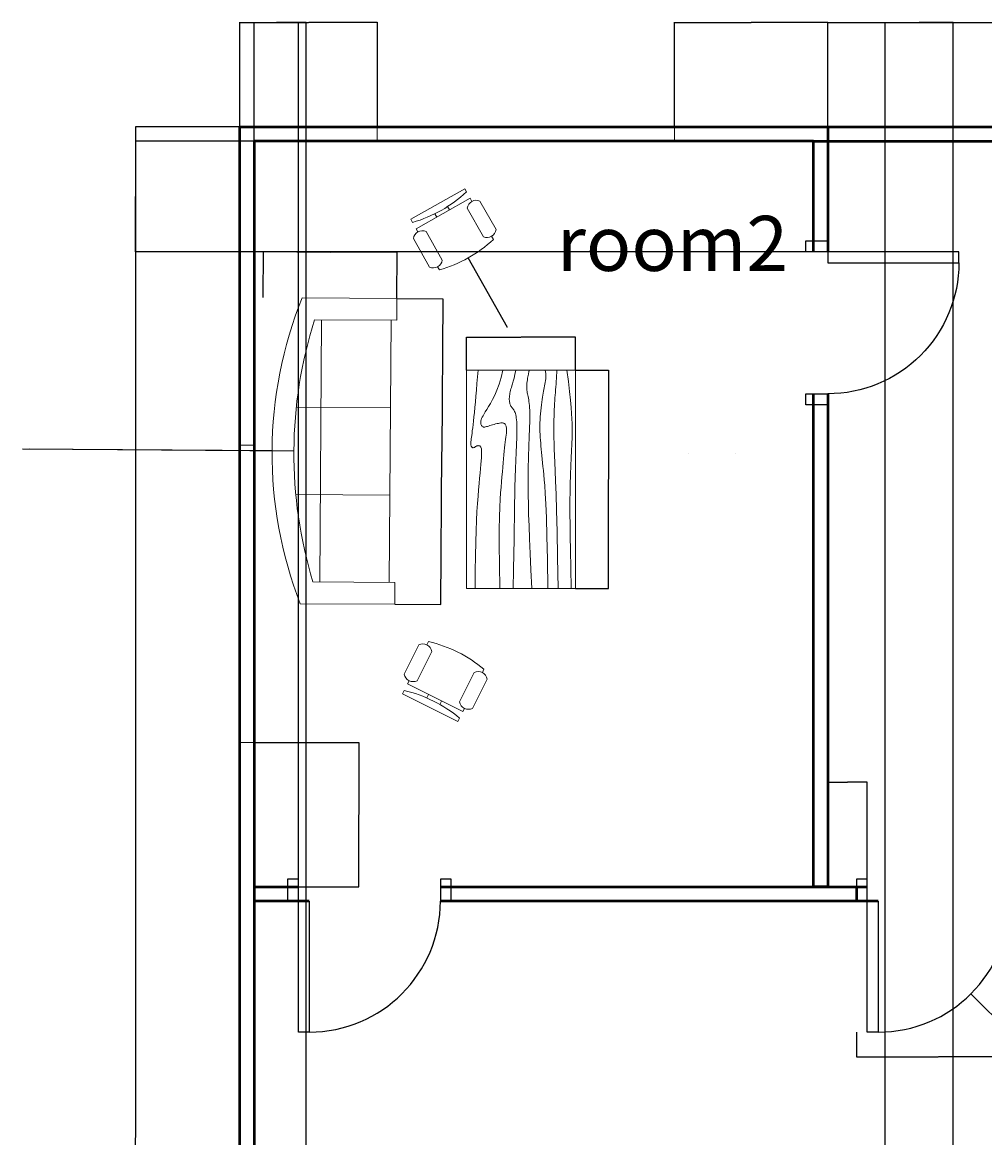
# Model space of a CAD drawing. Units: millimetres. Extents: x 756 to 17937, y 31 to 15590.
# Tile 2 of 6: x 756 to 7469, y 7810 to 15590. Entities that reach past the tile are written whole.
import ezdxf

# ---------------------------------------------------------------- set-up
doc = ezdxf.new("R2010")
doc.units = ezdxf.units.MM
for name, color, linetype, lineweight in [('A-ANNO-DIMS', 2, 'Continuous', 18), ('A-AREA-IDEN', 7, 'Continuous', 25), ('A-DOOR', 3, 'Continuous', 25), ('A-FURN', 8, 'Continuous', 18), ('A-GLAZ', 4, 'Continuous', 18), ('A-WALL', 7, 'Continuous', 50)]:
    doc.layers.add(name, color=color, linetype=linetype, lineweight=lineweight)
doc.styles.get("Standard").update_dxf_attribs({"font": 'arial.ttf'})
doc.dimstyles.get("Standard").update_dxf_attribs({"dimtxt": 0.18, "dimasz": 0.18, "dimexe": 0.18, "dimexo": 0.0625, "dimgap": 0.09, "dimtad": 0, "dimtih": 1, "dimtoh": 1, "dimdec": 4, "dimzin": 0, "dimdsep": 46, "dimtxsty": 'Standard', "dimcen": 0.09, "dimadec": 0, "dimazin": 0, "dimtfac": 1, "dimtdec": 4, "dimtofl": 0, "dimtmove": 0, "dimatfit": 3, "dimfxl": 1, "dimtolj": 1, "dimtzin": 0, "dimarcsym": 0})

# ---------------------------------------------------------------- blocks, each defined once
blk = doc.blocks.new('Sofa - Roundback 7 ft.')
for p, q in [((-12.00002, -32.4421), (-12.00003, -6.5971)), ((11.99997, -32.4421), (11.99998, -6.5971)), ((-36.000027, -34), (-36.000027, -11.4696)), ((35.99998, -34), (35.99998, -11.4696)), ((-35.999844, -13.3819), (35.9998, -13.3819)), ((-36.000027, -32.4421), (35.99998, -32.4421))]:
    blk.add_line(p, q)
for points in [[(-36.000027, -34), (-42.000027, -34), (-42.000027, -8)], [(41.99998, -8), (41.99998, -34), (35.99998, -34)]]:
    blk.add_lwpolyline(points)
for centre, radius, start, end in [((0, -114.25), 114.25, 68.43141, 111.5686), ((-0.00001, -127.1968), 121.1968, 72.72033, 107.2797)]:
    blk.add_arc(centre, radius, start, end)
blk = doc.blocks.new('Table - Rectangular Woodgrain 60 x 30 in.')
for p, q in [((0, 0), (0, -30)), ((60, 0), (0, 0)), ((60, -30), (60, 0)), ((0, -30), (60, -30))]:
    blk.add_line(p, q)
for points in [[(0, -2.4), (4.8155, -2.418), (9.0302, -2.4688), (12.709, -2.5477), (15.9167, -2.65), (18.7181, -2.7711), (21.1781, -2.9063), (23.3616, -3.0508), (25.3333, -3.2), (27.1477, -3.3495), (28.8172, -3.4958), (30.3437, -3.636), (31.7291, -3.7667), (32.9756, -3.8849), (34.0849, -3.9875), (35.059, -4.0714), (35.9, -4.1334), (36.6114, -4.1711), (37.2041, -4.1854), (37.6906, -4.1779), (38.0833, -4.15), (38.3948, -4.1034), (38.6375, -4.0396), (38.8239, -3.9602), (38.9666, -3.8667), (39.0764, -3.7608), (39.1573, -3.6448), (39.2116, -3.521), (39.2416, -3.3917), (39.2498, -3.2593), (39.2385, -3.1261), (39.21, -2.9944), (39.1666, -2.8667), (39.111, -2.7447), (39.0468, -2.6281), (38.978, -2.5163), (38.9083, -2.4083), (38.8418, -2.3035), (38.7823, -2.201), (38.7337, -2.1001), (38.7, -2), (38.6844, -1.9003), (38.6875, -1.8021), (38.7094, -1.707), (38.75, -1.6167), (38.8094, -1.5326), (38.8875, -1.4563), (38.9844, -1.3893), (39.1, -1.3333), (39.2351, -1.2896), (39.3937, -1.2583), (39.5804, -1.2396), (39.8, -1.2333), (40.057, -1.2396), (40.3562, -1.2583), (40.7023, -1.2896), (41.1, -1.3333), (41.5547, -1.3895), (42.0755, -1.4573), (42.6721, -1.5361), (43.3542, -1.625), (44.1316, -1.7233), (45.014, -1.8302), (46.0114, -1.9449), (47.1333, -2.0667), (48.3862, -2.1947), (49.7625, -2.3281), (51.2513, -2.4663), (52.8416, -2.6083), (54.5226, -2.7535), (56.2833, -2.9011), (58.1127, -3.0501), (60, -3.2)], [(0, -9.2), (6.5759, -9.0858), (11.9385, -9.0365), (16.2527, -9.0418), (19.6833, -9.0917), (22.3952, -9.1759), (24.5531, -9.2844), (26.322, -9.4069), (27.8666, -9.5333), (29.3241, -9.6553), (30.7203, -9.7719), (32.0532, -9.8837), (33.3208, -9.9917), (34.5213, -10.0965), (35.6526, -10.199), (36.7128, -10.2999), (37.7, -10.4), (38.6129, -10.4996), (39.4531, -10.5969), (40.223, -10.6895), (40.925, -10.775), (41.5613, -10.8512), (42.1344, -10.9156), (42.6465, -10.966), (43.1, -11), (43.4976, -11.0158), (43.8437, -11.0136), (44.143, -10.9942), (44.4, -10.9583), (44.6195, -10.9069), (44.8062, -10.8406), (44.9648, -10.7603), (45.1, -10.6667), (45.2155, -10.5598), (45.3114, -10.4365), (45.3871, -10.2929), (45.4416, -10.125), (45.4743, -9.929), (45.4844, -9.7011), (45.4709, -9.4371), (45.4333, -9.1333), (45.3716, -8.7883), (45.2896, -8.4104), (45.1919, -8.0107), (45.0833, -7.6), (44.9685, -7.1893), (44.8521, -6.7896), (44.7388, -6.4117), (44.6333, -6.0667), (44.54, -5.7628), (44.4614, -5.4979), (44.4001, -5.2675), (44.3583, -5.0667), (44.3384, -4.8909), (44.3427, -4.7354), (44.3736, -4.5956), (44.4333, -4.4667), (44.5236, -4.3453), (44.6427, -4.2333), (44.7884, -4.1339), (44.9583, -4.05), (45.1501, -3.9849), (45.3614, -3.9417), (45.59, -3.9234), (45.8333, -3.9333), (46.0915, -3.9749), (46.3734, -4.0531), (46.6906, -4.1736), (47.0542, -4.3417), (47.4756, -4.5629), (47.9661, -4.8427), (48.5372, -5.1866), (49.2, -5.6), (49.9676, -6.0844), (50.8594, -6.625), (51.8965, -7.2031), (53.1, -7.8), (54.491, -8.3969), (56.0906, -8.975), (57.9199, -9.5156), (60, -10)], [(0, -12.8), (5.1847, -12.9322), (9.6213, -13.0323), (13.3963, -13.1059), (16.5958, -13.1583), (19.3063, -13.1952), (21.614, -13.2219), (23.6054, -13.2439), (25.3666, -13.2667), (26.9728, -13.2947), (28.4531, -13.3281), (29.8256, -13.3663), (31.1083, -13.4083), (32.3191, -13.4535), (33.476, -13.501), (34.597, -13.5501), (35.7, -13.6), (36.7984, -13.6497), (37.8875, -13.6979), (38.9578, -13.743), (40, -13.7833), (41.0047, -13.8174), (41.9625, -13.8438), (42.864, -13.8607), (43.7, -13.8667), (44.4631, -13.8604), (45.1552, -13.8417), (45.7801, -13.8104), (46.3416, -13.7667), (46.8439, -13.7104), (47.2906, -13.6417), (47.6858, -13.5604), (48.0333, -13.4667), (48.3375, -13.3608), (48.6042, -13.2448), (48.8396, -13.121), (49.05, -12.9917), (49.2417, -12.8593), (49.4208, -12.7261), (49.5937, -12.5944), (49.7667, -12.4667), (49.9452, -12.3451), (50.1323, -12.2313), (50.3303, -12.1268), (50.5416, -12.0333), (50.7686, -11.9524), (51.0135, -11.8854), (51.2788, -11.8341), (51.5666, -11.8), (51.8785, -11.7843), (52.2116, -11.7865), (52.562, -11.8059), (52.926, -11.8417), (53.2998, -11.8931), (53.6795, -11.9594), (54.0614, -12.0397), (54.4416, -12.1333), (54.8223, -12.2401), (55.2293, -12.3625), (55.6942, -12.5037), (56.2489, -12.6667), (56.9251, -12.8547), (57.7545, -13.0708), (58.7689, -13.3182), (60, -13.6)], [(0, -18), (5.124, -17.7273), (9.6609, -17.5057), (13.6705, -17.3303), (17.2125, -17.1958), (20.3467, -17.0973), (23.1328, -17.0297), (25.6307, -16.9878), (27.9, -16.9667), (29.9928, -16.9617), (31.9302, -16.9703), (33.7254, -16.9907), (35.3917, -17.0208), (36.9423, -17.0588), (38.3906, -17.1026), (39.7499, -17.1503), (41.0333, -17.2), (42.2519, -17.2496), (43.4073, -17.2969), (44.4986, -17.3395), (45.525, -17.375), (46.4858, -17.4012), (47.3802, -17.4156), (48.2074, -17.416), (48.9667, -17.4), (49.6583, -17.3662), (50.2872, -17.3167), (50.8595, -17.2547), (51.3812, -17.1833), (51.8584, -17.1057), (52.2971, -17.025), (52.7034, -16.9443), (53.0833, -16.8667), (53.443, -16.7951), (53.789, -16.7313), (54.128, -16.6768), (54.4666, -16.6334), (54.8115, -16.6024), (55.1693, -16.5854), (55.5465, -16.5841), (55.95, -16.6), (56.3828, -16.6337), (56.8346, -16.6823), (57.2915, -16.7418), (57.7396, -16.8084), (58.165, -16.878), (58.5539, -16.9469), (58.8924, -17.0111), (59.1666, -17.0667), (59.3679, -17.1107), (59.5078, -17.1438), (59.6032, -17.1675), (59.6708, -17.1833), (59.7275, -17.193), (59.7901, -17.1979), (59.8753, -17.1998), (60, -17.2)], [(0, -22.4), (8.0098, -22.2501), (14.4094, -22.1011), (19.4168, -21.9535), (23.25, -21.8083), (26.1269, -21.6663), (28.2656, -21.5281), (29.884, -21.3947), (31.2, -21.2667), (32.3967, -21.1448), (33.5172, -21.0292), (34.5697, -20.9198), (35.5625, -20.8167), (36.5037, -20.7198), (37.4015, -20.6292), (38.2642, -20.5448), (39.1, -20.4667), (39.9164, -20.3951), (40.7187, -20.3313), (41.5117, -20.2768), (42.3, -20.2333), (43.0883, -20.2024), (43.8812, -20.1854), (44.6836, -20.1841), (45.5, -20.2), (46.3328, -20.234), (47.1747, -20.2844), (48.0163, -20.3488), (48.8479, -20.425), (49.66, -20.5106), (50.4429, -20.6031), (51.1872, -20.7004), (51.8833, -20.8), (52.5246, -20.8999), (53.1166, -20.9995), (53.6681, -21.0983), (54.1875, -21.1958), (54.6834, -21.2919), (55.1646, -21.3859), (55.6394, -21.4777), (56.1167, -21.5667), (56.6028, -21.6515), (57.0961, -21.7266), (57.5929, -21.7852), (58.0896, -21.8208), (58.5823, -21.8268), (59.0674, -21.7964), (59.5412, -21.723), (60, -21.6)], [(0, -25.2), (8.6355, -25.0504), (15.7026, -24.9031), (21.4049, -24.7606), (25.9458, -24.625), (29.529, -24.4988), (32.3578, -24.3844), (34.6359, -24.284), (36.5667, -24.2), (38.3213, -24.1341), (39.9417, -24.0854), (41.437, -24.0523), (42.8167, -24.0333), (44.0901, -24.0268), (45.2667, -24.0313), (46.3557, -24.0451), (47.3667, -24.0667), (48.309, -24.0947), (49.1928, -24.1287), (50.0284, -24.168), (50.826, -24.2125), (51.5959, -24.2617), (52.3483, -24.3151), (53.0935, -24.3725), (53.8417, -24.4334), (54.6009, -24.497), (55.3699, -24.561), (56.1454, -24.6226), (56.9239, -24.6792), (57.7021, -24.7279), (58.4764, -24.7662), (59.2435, -24.7911), (60, -24.8)], [(0, -28.8), (5.6867, -28.6681), (10.45, -28.5698), (14.407, -28.5012), (17.675, -28.4584), (20.3711, -28.4374), (22.6125, -28.4344), (24.5164, -28.4455), (26.2, -28.4667), (27.762, -28.4947), (29.2276, -28.5281), (30.6033, -28.5663), (31.8958, -28.6084), (33.1118, -28.6535), (34.2578, -28.7011), (35.3405, -28.7501), (36.3666, -28.8), (37.3443, -28.8497), (38.288, -28.8974), (39.2137, -28.9412), (40.1375, -28.9792), (41.0753, -29.0093), (42.0432, -29.0297), (43.0572, -29.0384), (44.1333, -29.0333), (45.2936, -29.0114), (46.5843, -28.9641), (48.0579, -28.8816), (49.7666, -28.7542), (51.7629, -28.5721), (54.0989, -28.3255), (56.8272, -28.0048), (60, -27.6)]]:
    blk.add_lwpolyline(points)
blk = doc.blocks.new('Chair - Desk')
for p, q in [((-8.5, 0), (-8.5, -1)), ((-8.5, 0), (8.5, 0)), ((8.5, 0), (8.5, -1)), ((-8.5, -3), (-8.5, -4)), ((-8.5, -3), (8.5, -3)), ((-2, -3), (-2, -1.9355)), ((2, -1.9576), (2, -3)), ((8.5, -3), (8.5, -4)), ((-10.5, -5), (-10.5, -14)), ((-6.5, -14), (-6.5, -5)), ((6.5, -5), (6.5, -14)), ((10.5, -14), (10.5, -5)), ((-8.5, -15), (-8.5, -16)), ((8.5, -15), (8.5, -16))]:
    blk.add_line(p, q)
for centre, radius, start, end in [((0, 34.625), 36.625, 256.5803, 283.4197), ((-8.5, -6.5), 2.5, 36.8699, 143.1301), ((8.5, -6.5), 2.5, 36.8699, 143.1301), ((-8.5, -12.5), 2.5, 216.8699, 323.1301), ((8.5, -12.5), 2.5, 216.8699, 323.1301), ((0, 19.625), 36.625, 256.5803, 283.4197)]:
    blk.add_arc(centre, radius, start, end)
blk = doc.blocks.new('DOOR-SINGLE-914')
for p, q in [((76.2, 1066.8), (0, 1066.8)), ((0, 1066.8), (0, 914.4)), ((76.2, 914.4), (76.2, 1066.8)), ((1143, 1066.8), (1066.8, 1066.8)), ((1066.8, 1066.8), (1066.8, 914.4)), ((1143, 914.4), (1143, 1066.8)), ((0, 914.4), (76.2, 914.4)), ((76.2, 914.4), (152.4, 914.4)), ((76.2, 0), (76.2, 914.4)), ((152.4, 914.4), (152.4, 0)), ((1066.8, 914.4), (1143, 914.4)), ((152.4, 0), (76.2, 0))]:
    blk.add_line(p, q)
blk.add_arc((152.4, 914.4), 914.4, 270, 0)
blk = doc.blocks.new('WIN-2073')
for p, q in [((0, 100), (0, 0)), ((2072.9, 100), (0, 100)), ((2072.9, 0), (2072.9, 100)), ((0, 0), (2072.9, 0))]:
    blk.add_line(p, q)
blk = doc.blocks.new('*D15')
at = {"layer": 'A-ANNO-DIMS', "color": 0, "lineweight": -2, "transparency": 16777216}
for p, q in [((6574.2, 8546.1), (6574.2, 8374.6)), ((7717.2, 8546.1), (7717.2, 8374.6)), ((6574.4, 8374.8), (7144.1, 8374.8)), ((7717, 8374.8), (7147.3, 8374.8))]:
    blk.add_line(p, q, dxfattribs=at)
at = {"layer": 'A-ANNO-DIMS', "color": 0, "transparency": 16777216}
for points in [[(6574.4, 8374.8), (6574.4, 8374.7), (6574.2, 8374.8)], [(7717, 8374.8), (7717, 8374.7), (7717.2, 8374.8)]]:
    blk.add_solid(points, dxfattribs=at)
at = {"layer": 'Defpoints', "color": 0, "transparency": 16777216}
for p in [(6574.2, 8546.2), (7717.2, 8546.2), (7717.2, 8374.8)]:
    blk.add_point(p, dxfattribs=at)
at = {"layer": 'A-ANNO-DIMS', "color": 0, "transparency": 16777216, "insert": (7145.7, 8374.8), "char_height": 0.18, "attachment_point": 5}
blk.add_mtext('\\A1;SINGLE DOOR 1143 TYP.', dxfattribs=at)
blk = doc.blocks.new('*D27')
at = {"layer": 'A-ANNO-DIMS', "color": 0, "lineweight": -2, "transparency": 16777216}
for p, q in [((3368.6, 13664), (3688.7, 13661.9)), ((3688.6, 13661.7), (3681.7, 12595.3)), ((3674.8, 11528.5), (3681.7, 12594.9)), ((3354.8, 11530.4), (3675, 11528.3))]:
    blk.add_line(p, q, dxfattribs=at)
at = {"layer": 'A-ANNO-DIMS', "color": 0, "transparency": 16777216}
for points in [[(3688.5, 13661.7), (3688.6, 13661.7), (3688.6, 13661.9)], [(3674.8, 11528.5), (3674.8, 11528.5), (3674.8, 11528.3)]]:
    blk.add_solid(points, dxfattribs=at)
at = {"layer": 'Defpoints', "color": 0, "transparency": 16777216}
for p in [(3368.5, 13664), (3688.6, 13661.9), (3354.8, 11530.4)]:
    blk.add_point(p, dxfattribs=at)
at = {"layer": 'A-ANNO-DIMS', "color": 0, "transparency": 16777216, "insert": (3681.7, 12595.1), "char_height": 0.18, "attachment_point": 5}
blk.add_mtext('\\A1;SOFA 2134', dxfattribs=at)
blk = doc.blocks.new('*D28')
at = {"layer": 'A-ANNO-DIMS', "color": 0, "lineweight": -2, "transparency": 16777216}
for p, q in [((2437.2, 13670), (2439.3, 13990.2)), ((2439.4, 13990), (2904.7, 13987)), ((3370.4, 13984), (2905.2, 13987)), ((3368.5, 13664), (3370.6, 13984.2))]:
    blk.add_line(p, q, dxfattribs=at)
at = {"layer": 'A-ANNO-DIMS', "color": 0, "transparency": 16777216}
for points in [[(2439.4, 13990), (2439.4, 13990), (2439.3, 13990)], [(3370.4, 13984), (3370.4, 13984), (3370.6, 13984)]]:
    blk.add_solid(points, dxfattribs=at)
at = {"layer": 'Defpoints', "color": 0, "transparency": 16777216}
for p in [(2439.3, 13990), (2437.2, 13670), (3368.5, 13664)]:
    blk.add_point(p, dxfattribs=at)
at = {"layer": 'A-ANNO-DIMS', "color": 0, "transparency": 16777216, "insert": (2904.9, 13987), "char_height": 0.18, "attachment_point": 5}
blk.add_mtext('\\A1;931', dxfattribs=at)
blk = doc.blocks.new('*D29')
at = {"layer": 'A-ANNO-DIMS', "color": 0, "lineweight": -2, "transparency": 16777216}
for p, q in [((4616, 13164.1), (4844.7, 13164.1)), ((4844.5, 13163.9), (4844.5, 12402.3)), ((4844.5, 11640.3), (4844.5, 12401.9)), ((4616, 11640.1), (4844.7, 11640.1))]:
    blk.add_line(p, q, dxfattribs=at)
at = {"layer": 'A-ANNO-DIMS', "color": 0, "transparency": 16777216}
for points in [[(4844.5, 13163.9), (4844.5, 13163.9), (4844.5, 13164.1)], [(4844.5, 11640.3), (4844.5, 11640.3), (4844.5, 11640.1)]]:
    blk.add_solid(points, dxfattribs=at)
at = {"layer": 'Defpoints', "color": 0, "transparency": 16777216}
for p in [(4615.9, 13164.1), (4844.5, 13164.1), (4615.9, 11640.1)]:
    blk.add_point(p, dxfattribs=at)
at = {"layer": 'A-ANNO-DIMS', "color": 0, "transparency": 16777216, "insert": (4844.5, 12402.1), "char_height": 0.18, "attachment_point": 5}
blk.add_mtext('\\A1;LOW TABLE 1524', dxfattribs=at)
blk = doc.blocks.new('*D30')
at = {"layer": 'A-ANNO-DIMS', "color": 0, "lineweight": -2, "transparency": 16777216}
for p, q in [((3853.9, 13164.1), (3853.9, 13392.9)), ((3854.1, 13392.7), (4234.6, 13392.7)), ((4615.7, 13392.7), (4235.2, 13392.7)), ((4615.9, 13164.1), (4615.9, 13392.9))]:
    blk.add_line(p, q, dxfattribs=at)
at = {"layer": 'A-ANNO-DIMS', "color": 0, "transparency": 16777216}
for points in [[(3854.1, 13392.7), (3854.1, 13392.6), (3853.9, 13392.7)], [(4615.7, 13392.7), (4615.7, 13392.6), (4615.9, 13392.7)]]:
    blk.add_solid(points, dxfattribs=at)
at = {"layer": 'Defpoints', "color": 0, "transparency": 16777216}
for p in [(3853.9, 13392.7), (3853.9, 13164.1), (4615.9, 13164.1)]:
    blk.add_point(p, dxfattribs=at)
at = {"layer": 'A-ANNO-DIMS', "color": 0, "transparency": 16777216, "insert": (4234.9, 13392.7), "char_height": 0.18, "attachment_point": 5}
blk.add_mtext('\\A1;762', dxfattribs=at)
blk = doc.blocks.new('*D44')
at = {"layer": 'A-ANNO-DIMS', "color": 0, "lineweight": -2, "transparency": 16777216}
for p, q in [((2274.1, 14860.2), (1544.7, 14860.2)), ((1544.9, 14860), (1544.9, 7810.4)), ((1544.9, 760.4), (1544.9, 7810)), ((2274.1, 760.2), (1544.7, 760.2))]:
    blk.add_line(p, q, dxfattribs=at)
at = {"layer": 'A-ANNO-DIMS', "color": 0, "transparency": 16777216}
for points in [[(1544.8, 14860), (1544.9, 14860), (1544.9, 14860.2)], [(1544.8, 760.4), (1544.9, 760.4), (1544.9, 760.2)]]:
    blk.add_solid(points, dxfattribs=at)
at = {"layer": 'Defpoints', "color": 0, "transparency": 16777216}
for p in [(1544.9, 14860.2), (2274.1, 14860.2), (2274.1, 760.2)]:
    blk.add_point(p, dxfattribs=at)
at = {"layer": 'A-ANNO-DIMS', "color": 0, "transparency": 16777216, "insert": (1544.9, 7810.2), "char_height": 0.18, "attachment_point": 5}
blk.add_mtext('\\A1;14100', dxfattribs=at)
blk = doc.blocks.new('*D53')
at = {"layer": 'A-ANNO-DIMS', "color": 0, "lineweight": -2, "transparency": 16777216}
for p, q in [((2274.1, 14860.2), (2274.1, 15589.6)), ((2274.3, 15589.4), (2753, 15589.4)), ((3232.4, 15589.4), (2753.7, 15589.4)), ((3232.6, 14860.2), (3232.6, 15589.6))]:
    blk.add_line(p, q, dxfattribs=at)
at = {"layer": 'A-ANNO-DIMS', "color": 0, "transparency": 16777216}
for points in [[(2274.3, 15589.5), (2274.3, 15589.4), (2274.1, 15589.4)], [(3232.4, 15589.5), (3232.4, 15589.4), (3232.6, 15589.4)]]:
    blk.add_solid(points, dxfattribs=at)
at = {"layer": 'Defpoints', "color": 0, "transparency": 16777216}
for p in [(3232.6, 15589.4), (2274.1, 14860.2), (3232.6, 14860.2)]:
    blk.add_point(p, dxfattribs=at)
at = {"layer": 'A-ANNO-DIMS', "color": 0, "transparency": 16777216, "insert": (2753.3, 15589.4), "char_height": 0.18, "attachment_point": 5}
blk.add_mtext('\\A1;958.5', dxfattribs=at)
blk = doc.blocks.new('*D54')
at = {"layer": 'A-ANNO-DIMS', "color": 0, "lineweight": -2, "transparency": 16777216}
for p, q in [((5305.5, 14860.2), (5305.5, 15589.6)), ((5305.7, 15589.4), (5839.3, 15589.4)), ((6373.9, 15589.4), (5840.3, 15589.4)), ((6374.1, 14860.2), (6374.1, 15589.6))]:
    blk.add_line(p, q, dxfattribs=at)
at = {"layer": 'A-ANNO-DIMS', "color": 0, "transparency": 16777216}
for points in [[(5305.7, 15589.5), (5305.7, 15589.4), (5305.5, 15589.4)], [(6373.9, 15589.5), (6373.9, 15589.4), (6374.1, 15589.4)]]:
    blk.add_solid(points, dxfattribs=at)
at = {"layer": 'Defpoints', "color": 0, "transparency": 16777216}
for p in [(6374.1, 15589.4), (5305.5, 14860.2), (6374.1, 14860.2)]:
    blk.add_point(p, dxfattribs=at)
at = {"layer": 'A-ANNO-DIMS', "color": 0, "transparency": 16777216, "insert": (5839.8, 15589.4), "char_height": 0.18, "attachment_point": 5}
blk.add_mtext('\\A1;1068.6', dxfattribs=at)
blk = doc.blocks.new('*D55')
at = {"layer": 'A-ANNO-DIMS', "color": 0, "lineweight": -2, "transparency": 16777216}
for p, q in [((6374.1, 14860.2), (6374.1, 15589.6)), ((6374.3, 15589.4), (7637, 15589.4)), ((8900.6, 15589.4), (7637.9, 15589.4)), ((8900.8, 14860.2), (8900.8, 15589.6))]:
    blk.add_line(p, q, dxfattribs=at)
at = {"layer": 'A-ANNO-DIMS', "color": 0, "transparency": 16777216}
for points in [[(6374.3, 15589.5), (6374.3, 15589.4), (6374.1, 15589.4)], [(8900.6, 15589.5), (8900.6, 15589.4), (8900.8, 15589.4)]]:
    blk.add_solid(points, dxfattribs=at)
at = {"layer": 'Defpoints', "color": 0, "transparency": 16777216}
for p in [(8900.8, 15589.4), (6374.1, 14860.2), (8900.8, 14860.2)]:
    blk.add_point(p, dxfattribs=at)
at = {"layer": 'A-ANNO-DIMS', "color": 0, "transparency": 16777216, "insert": (7637.4, 15589.4), "char_height": 0.18, "attachment_point": 5}
blk.add_mtext('\\A1;2526.6', dxfattribs=at)
blk = doc.blocks.new('*D63')
at = {"layer": 'A-ANNO-DIMS', "color": 0, "lineweight": -2, "transparency": 16777216}
for p, q in [((2374.1, 860.2), (2374.1, 15589.6)), ((2374.3, 15589.4), (2554.6, 15589.4)), ((2735.7, 15589.4), (2555.4, 15589.4)), ((2735.9, 760.2), (2735.9, 15589.6))]:
    blk.add_line(p, q, dxfattribs=at)
at = {"layer": 'A-ANNO-DIMS', "color": 0, "transparency": 16777216}
for points in [[(2374.3, 15589.5), (2374.3, 15589.4), (2374.1, 15589.4)], [(2735.7, 15589.5), (2735.7, 15589.4), (2735.9, 15589.4)]]:
    blk.add_solid(points, dxfattribs=at)
at = {"layer": 'Defpoints', "color": 0, "transparency": 16777216}
for p in [(2735.9, 15589.4), (2374.1, 860.2), (2735.9, 760.2)]:
    blk.add_point(p, dxfattribs=at)
at = {"layer": 'A-ANNO-DIMS', "color": 0, "transparency": 16777216, "insert": (2555, 15589.4), "char_height": 0.18, "attachment_point": 5}
blk.add_mtext('\\A1;361.8', dxfattribs=at)
blk = doc.blocks.new('*D64')
at = {"layer": 'A-ANNO-DIMS', "color": 0, "lineweight": -2, "transparency": 16777216}
for p, q in [((6774.1, 860.2), (6774.1, 15589.6)), ((6774.3, 15589.4), (7011.6, 15589.4)), ((7249.8, 15589.4), (7012.4, 15589.4)), ((7250, 860.2), (7250, 15589.6))]:
    blk.add_line(p, q, dxfattribs=at)
at = {"layer": 'A-ANNO-DIMS', "color": 0, "transparency": 16777216}
for points in [[(6774.3, 15589.5), (6774.3, 15589.4), (6774.1, 15589.4)], [(7249.8, 15589.5), (7249.8, 15589.4), (7250, 15589.4)]]:
    blk.add_solid(points, dxfattribs=at)
at = {"layer": 'Defpoints', "color": 0, "transparency": 16777216}
for p in [(7250, 15589.4), (6774.1, 860.2), (7250, 860.2)]:
    blk.add_point(p, dxfattribs=at)
at = {"layer": 'A-ANNO-DIMS', "color": 0, "transparency": 16777216, "insert": (7012, 15589.4), "char_height": 0.18, "attachment_point": 5}
blk.add_mtext('\\A1;475.9', dxfattribs=at)
blk = doc.blocks.new('*D67')
at = {"layer": 'A-ANNO-DIMS', "color": 0, "lineweight": -2, "transparency": 16777216}
for p, q in [((2374.2, 10566.3), (3103.5, 10566.3)), ((3103.4, 10566.1), (3103.4, 10063.4)), ((3103.4, 9560.4), (3103.4, 10063.1)), ((2374.2, 9560.2), (3103.5, 9560.2))]:
    blk.add_line(p, q, dxfattribs=at)
at = {"layer": 'A-ANNO-DIMS', "color": 0, "transparency": 16777216}
for points in [[(3103.3, 10566.1), (3103.4, 10566.1), (3103.4, 10566.3)], [(3103.3, 9560.4), (3103.4, 9560.4), (3103.4, 9560.2)]]:
    blk.add_solid(points, dxfattribs=at)
at = {"layer": 'Defpoints', "color": 0, "transparency": 16777216}
for p in [(2374.1, 10566.3), (2374.1, 9560.2), (3103.4, 9560.2)]:
    blk.add_point(p, dxfattribs=at)
at = {"layer": 'A-ANNO-DIMS', "color": 0, "transparency": 16777216, "insert": (3103.4, 10063.3), "char_height": 0.18, "attachment_point": 5}
blk.add_mtext('\\A1;1006.1', dxfattribs=at)
blk = doc.blocks.new('*D69')
at = {"layer": 'A-ANNO-DIMS', "color": 0, "lineweight": -2, "transparency": 16777216}
for p, q in [((6274.1, 14760.2), (1544.7, 14760.2)), ((1544.9, 14760), (1544.9, 14374.8)), ((1544.9, 13989.2), (1544.9, 14374.4)), ((6374.1, 13989), (1544.7, 13989))]:
    blk.add_line(p, q, dxfattribs=at)
at = {"layer": 'A-ANNO-DIMS', "color": 0, "transparency": 16777216}
for points in [[(1544.8, 14760), (1544.9, 14760), (1544.9, 14760.2)], [(1544.8, 13989.2), (1544.9, 13989.2), (1544.9, 13989)]]:
    blk.add_solid(points, dxfattribs=at)
at = {"layer": 'Defpoints', "color": 0, "transparency": 16777216}
for p in [(6274.1, 14760.2), (1544.9, 13989), (6374.1, 13989)]:
    blk.add_point(p, dxfattribs=at)
at = {"layer": 'A-ANNO-DIMS', "color": 0, "transparency": 16777216, "insert": (1544.9, 14374.6), "char_height": 0.18, "attachment_point": 5}
blk.add_mtext('\\A1;771.2', dxfattribs=at)
blk = doc.blocks.new('*D70')
at = {"layer": 'A-ANNO-DIMS', "color": 0, "lineweight": -2, "transparency": 16777216}
for p, q in [((2374.1, 9560.2), (2374.1, 15589.6)), ((2374.3, 15589.4), (2527.4, 15589.4)), ((2681.4, 15589.4), (2528.3, 15589.4)), ((2681.6, 9560.2), (2681.6, 15589.6))]:
    blk.add_line(p, q, dxfattribs=at)
at = {"layer": 'A-ANNO-DIMS', "color": 0, "transparency": 16777216}
for points in [[(2374.3, 15589.5), (2374.3, 15589.4), (2374.1, 15589.4)], [(2681.4, 15589.5), (2681.4, 15589.4), (2681.6, 15589.4)]]:
    blk.add_solid(points, dxfattribs=at)
at = {"layer": 'Defpoints', "color": 0, "transparency": 16777216}
for p in [(2681.6, 15589.4), (2374.1, 9560.2), (2681.6, 9560.2)]:
    blk.add_point(p, dxfattribs=at)
at = {"layer": 'A-ANNO-DIMS', "color": 0, "transparency": 16777216, "insert": (2527.8, 15589.4), "char_height": 0.18, "attachment_point": 5}
blk.add_mtext('\\A1;307.44', dxfattribs=at)
blk = doc.blocks.new('*D71')
at = {"layer": 'A-ANNO-DIMS', "color": 0, "lineweight": -2, "transparency": 16777216}
for p, q in [((6374.1, 9560.2), (6374.1, 10289.6)), ((6374.3, 10289.4), (6511.8, 10289.4)), ((6650.2, 10289.4), (6512.7, 10289.4)), ((6650.4, 9560.2), (6650.4, 10289.6))]:
    blk.add_line(p, q, dxfattribs=at)
at = {"layer": 'A-ANNO-DIMS', "color": 0, "transparency": 16777216}
for points in [[(6374.3, 10289.5), (6374.3, 10289.4), (6374.1, 10289.4)], [(6650.2, 10289.5), (6650.2, 10289.4), (6650.4, 10289.4)]]:
    blk.add_solid(points, dxfattribs=at)
at = {"layer": 'Defpoints', "color": 0, "transparency": 16777216}
for p in [(6650.4, 10289.4), (6374.1, 9560.2), (6650.4, 9560.2)]:
    blk.add_point(p, dxfattribs=at)
at = {"layer": 'A-ANNO-DIMS', "color": 0, "transparency": 16777216, "insert": (6512.2, 10289.4), "char_height": 0.18, "attachment_point": 5}
blk.add_mtext('\\A1;276.27', dxfattribs=at)
blk = doc.blocks.new('*D78')
at = {"layer": 'A-ANNO-DIMS', "color": 0, "lineweight": -2, "transparency": 16777216}
for p, q in [((6726.5, 9460.6), (6726.7, 9460.6)), ((6726.6, 9460.5), (6726.6, 9460.7)), ((7761.1, 8426.1), (7373.3, 8813.9)), ((7761.3, 8426.1), (7761.1, 8426.1))]:
    blk.add_line(p, q, dxfattribs=at)
at = {"layer": 'A-ANNO-DIMS', "color": 0, "transparency": 16777216}
blk.add_solid([(7373.3, 8813.9), (7373.3, 8813.9), (7373.2, 8814)], dxfattribs=at)
at = {"layer": 'Defpoints', "color": 0, "transparency": 16777216}
for p in [(6726.6, 9460.6), (7373.2, 8814)]:
    blk.add_point(p, dxfattribs=at)
at = {"layer": 'A-ANNO-DIMS', "color": 0, "transparency": 16777216, "insert": (7762, 8426.1), "char_height": 0.18, "attachment_point": 5}
blk.add_mtext('\\A1;5X R914.4', dxfattribs=at)
blk = doc.blocks.new('*D79')
at = {"layer": 'A-ANNO-DIMS', "color": 0, "lineweight": -2, "transparency": 16777216}
for p, q in [((756.9, 12614), (2497.9, 12602.8)), ((5399.9, 12583.9), (5399.9, 12584.1)), ((5399.9, 12584), (5400, 12584))]:
    blk.add_line(p, q, dxfattribs=at)
at = {"layer": 'A-ANNO-DIMS', "color": 0, "transparency": 16777216}
blk.add_solid([(2497.9, 12602.8), (2497.9, 12602.7), (2498.1, 12602.7)], dxfattribs=at)
at = {"layer": 'Defpoints', "color": 0, "transparency": 16777216}
for p in [(2498.1, 12602.7), (5399.9, 12584)]:
    blk.add_point(p, dxfattribs=at)
at = {"layer": 'A-ANNO-DIMS', "color": 0, "transparency": 16777216, "insert": (756.5, 12614), "char_height": 0.18, "attachment_point": 5}
blk.add_mtext('\\A1;R2902', dxfattribs=at)
blk = doc.blocks.new('*D80')
at = {"layer": 'A-ANNO-DIMS', "color": 0, "lineweight": -2, "transparency": 16777216}
for p, q in [((803.5, 12613.7), (2650.3, 12601.8)), ((5728.7, 12581.9), (5728.9, 12581.9)), ((5728.8, 12581.8), (5728.8, 12582))]:
    blk.add_line(p, q, dxfattribs=at)
at = {"layer": 'A-ANNO-DIMS', "color": 0, "transparency": 16777216}
blk.add_solid([(2650.3, 12601.8), (2650.3, 12601.7), (2650.5, 12601.8)], dxfattribs=at)
at = {"layer": 'Defpoints', "color": 0, "transparency": 16777216}
for p in [(2650.5, 12601.8), (5728.8, 12581.9)]:
    blk.add_point(p, dxfattribs=at)
at = {"layer": 'A-ANNO-DIMS', "color": 0, "transparency": 16777216, "insert": (802.9, 12613.7), "char_height": 0.18, "attachment_point": 5}
blk.add_mtext('\\A1;R3078.4', dxfattribs=at)
blk = doc.blocks.new('*D81')
at = {"layer": 'A-ANNO-DIMS', "color": 0, "lineweight": -2, "transparency": 16777216}
for p, q in [((3408.6, 14756.4), (3408.8, 14756.4)), ((3408.7, 14756.3), (3408.7, 14756.5)), ((4140.9, 13460.5), (3866.4, 13946.3)), ((4141.1, 13460.5), (4140.9, 13460.5))]:
    blk.add_line(p, q, dxfattribs=at)
at = {"layer": 'A-ANNO-DIMS', "color": 0, "transparency": 16777216}
blk.add_solid([(3866.5, 13946.3), (3866.4, 13946.3), (3866.3, 13946.5)], dxfattribs=at)
at = {"layer": 'Defpoints', "color": 0, "transparency": 16777216}
for p in [(3408.7, 14756.4), (3866.3, 13946.5)]:
    blk.add_point(p, dxfattribs=at)
at = {"layer": 'A-ANNO-DIMS', "color": 0, "transparency": 16777216, "insert": (4141.8, 13460.5), "char_height": 0.18, "attachment_point": 5}
blk.add_mtext('\\A1;6X R930.3', dxfattribs=at)

msp = doc.modelspace()

# ---------------------------------------------------------------- linework, layer by layer
at = {"layer": 'A-WALL'}
for p, q in [((2274.114, 9560.181), (2274.114, 14860.181)), ((2274.114, 14860.181), (6274.114, 14860.181)), ((6274.114, 14860.181), (6374.114, 14860.181)), ((6374.114, 14860.181), (6374.114, 13989.02)), ((6374.114, 14860.181), (11974.114, 14860.181)), ((6274.114, 14760.181), (2374.114, 14760.181)), ((2374.114, 14760.181), (2374.114, 9460.181)), ((6274.114, 14760.181), (11974.114, 14760.181)), ((6274.114, 13989.02), (6274.114, 14760.181)), ((6274.114, 9560.181), (6274.114, 12998.42)), ((6374.114, 12998.42), (6374.114, 9560.181)), ((2274.114, 4260.181), (2274.114, 9560.181)), ((2374.114, 9560.181), (2681.552, 9560.181)), ((3672.152, 9560.181), (6274.114, 9560.181)), ((6274.114, 9560.181), (6374.114, 9560.181)), ((6374.114, 9560.181), (6274.114, 9560.181)), ((6374.114, 9560.181), (6574.114, 9560.181)), ((6574.114, 9560.181), (6574.114, 9460.181)), ((6574.114, 9560.181), (6650.385, 9560.181)), ((2474.114, 9460.181), (2374.114, 9460.181)), ((2374.114, 9460.181), (2374.114, 4260.181)), ((2574.114, 9460.181), (2474.114, 9460.181)), ((2674.114, 9460.181), (2574.114, 9460.181)), ((2757.752, 9460.181), (2674.114, 9460.181)), ((6574.114, 9460.181), (3672.152, 9460.181)), ((6726.585, 9460.181), (6574.114, 9460.181))]:
    msp.add_line(p, q, dxfattribs=at)

# ---------------------------------------------------------------- block references
at = {"layer": 'A-DOOR', "extrusion": (0, 0, -1), "zscale": -1, "rotation": 270}
msp.add_blockref('DOOR-SINGLE-914', (-7289.2, 14065.22), dxfattribs=at)
msp.add_blockref('DOOR-SINGLE-914', (-7289.2, 14065.22), dxfattribs=at)
at = {"layer": 'A-DOOR'}
for p in [(2605.352, 8546.598), (6574.185, 8546.202)]:
    msp.add_blockref('DOOR-SINGLE-914', p, dxfattribs=at)
at = {"layer": 'A-FURN'}
for name, p, xscale, yscale, zscale, rotation in [('Chair - Desk', (3653.911, 14322.417), 25.39999999999999, 25.39999999999999, 25.39999999999999, 29.46931187105593), ('Sofa - Roundback 7 ft.', (2498.057, 12602.75), 25.4, 25.4, 25.4, 89.63054149427417), ('Table - Rectangular Woodgrain 60 x 30 in.', (3853.914, 11640.079), 25.4, 25.4, 25.4, 90), ('Chair - Desk', (3601.546, 10810.263), 25.4, 25.4, 25.4, 153.4349488229218)]:
    msp.add_blockref(name, p, dxfattribs=dict(at, xscale=xscale, yscale=yscale, zscale=zscale, rotation=rotation))
at = {"layer": 'A-GLAZ'}
msp.add_blockref('WIN-2073', (3232.577, 14760.181), dxfattribs=at)
at = {"layer": 'A-GLAZ', "rotation": 90.00000000000003}
msp.add_blockref('WIN-2073', (2374.113, 10566.322), dxfattribs=at)

# ---------------------------------------------------------------- texts
at = {"layer": 'A-AREA-IDEN', "insert": (4484.13, 14239.536), "char_height": 383.8245, "attachment_point": 1}
msp.add_mtext_dynamic_manual_height_columns('room2', width=5870.21244, gutter_width=1919.122, heights=[0], dxfattribs=at)

# ---------------------------------------------------------------- dimensions: what is measured, and where the dimension line sits
at = {"layer": 'A-ANNO-DIMS'}
for base, p1, p2, override, picture, middle in [((3232.577, 15589.431), (2274.114, 14860.181), (3232.577, 14860.181), {"dimdec": 1, "dimlfac": 1, "dimrnd": 0, "dimzin": 0, "dimdsep": 46, "dimlunit": 2}, '*D53', (2753.345, 15589.431)), ((2735.923, 15589.431), (2374.114, 860.181), (2735.923, 760.181), {"dimdec": 1, "dimlfac": 1, "dimrnd": 0, "dimzin": 0, "dimdsep": 46, "dimlunit": 2}, '*D63', (2555.018, 15589.431)), ((2681.552, 15589.431), (2374.114, 9560.181), (2681.552, 9560.181), {"dimdec": 2, "dimlfac": 1, "dimrnd": 0, "dimzin": 0, "dimdsep": 46, "dimlunit": 2}, '*D70', (2527.833, 15589.431)), ((6374.114, 15589.431), (5305.481, 14860.181), (6374.114, 14860.181), {"dimdec": 1, "dimlfac": 1, "dimrnd": 0, "dimzin": 0, "dimdsep": 46, "dimlunit": 2}, '*D54', (5839.797, 15589.431)), ((8900.754, 15589.431), (6374.114, 14860.181), (8900.754, 14860.181), {"dimdec": 1, "dimlfac": 1, "dimrnd": 0, "dimzin": 0, "dimdsep": 46, "dimlunit": 2}, '*D55', (7637.434, 15589.431)), ((7249.967, 15589.431), (6774.114, 860.181), (7249.967, 860.181), {"dimdec": 1, "dimlfac": 1, "dimrnd": 0, "dimzin": 0, "dimdsep": 46, "dimlunit": 2}, '*D64', (7012.041, 15589.431)), ((6650.385, 10289.431), (6374.114, 9560.181), (6650.385, 9560.181), {"dimdec": 2, "dimlfac": 1, "dimrnd": 0, "dimzin": 0, "dimdsep": 46, "dimlunit": 2}, '*D71', (6512.25, 10289.431))]:
    dim = msp.add_linear_dim(base=base, p1=p1, p2=p2, dimstyle='Standard', override=override, dxfattribs=at)
    dim.commit()
    dim.dimension.update_dxf_attribs({"geometry": picture, "text_midpoint": middle})
for base, p1, p2, angle, override, picture, middle in [((1544.864, 14860.181), (2274.114, 760.181), (2274.114, 14860.181), 90, {"dimdec": 0, "dimlfac": 1, "dimrnd": 0, "dimzin": 0, "dimdsep": 46, "dimlunit": 2}, '*D44', (1544.864, 7810.181)), ((1544.864, 13989.02), (6274.114, 14760.181), (6374.114, 13989.02), 90, {"dimdec": 1, "dimlfac": 1, "dimrnd": 0, "dimzin": 0, "dimdsep": 46, "dimlunit": 2}, '*D69', (1544.864, 14374.6)), ((2439.268, 13989.998), (3368.518, 13663.959), (2437.204, 13669.965), 179.6305415, {"dimdec": 0, "dimlfac": 1, "dimrnd": 0, "dimzin": 0, "dimdsep": 46, "dimlunit": 2}, '*D28', (2904.925, 13986.995)), ((3853.914, 13392.679), (4615.914, 13164.079), (3853.914, 13164.079), 180, {"dimdec": 0, "dimlfac": 1, "dimrnd": 0, "dimzin": 0, "dimdsep": 46, "dimlunit": 2}, '*D30', (4234.914, 13392.679)), ((3103.364, 9560.181), (2374.114, 10566.322), (2374.114, 9560.181), 270, {"dimdec": 1, "dimlfac": 1, "dimrnd": 0, "dimzin": 0, "dimdsep": 46, "dimlunit": 2}, '*D67', (3103.364, 10063.251))]:
    dim = msp.add_linear_dim(base=base, p1=p1, p2=p2, angle=angle, dimstyle='Standard', override=override, dxfattribs=at)
    dim.commit()
    dim.dimension.update_dxf_attribs({"geometry": picture, "text_midpoint": middle})
for center, mpoint, text, picture, middle in [((3408.682, 14756.399), (3866.338, 13946.483), '6X <>', '*D81', (4141.785, 13460.534)), ((6726.585, 9460.602), (7373.164, 8814.024), '5X <>', '*D78', (7761.964, 8426.077))]:
    dim = msp.add_radius_dim(center=center, mpoint=mpoint, text=text, dimstyle='Standard', override={"dimdec": 1, "dimlfac": 1, "dimrnd": 0, "dimzin": 0, "dimdsep": 46, "dimlunit": 2}, dxfattribs=at)
    dim.commit()
    dim.dimension.update_dxf_attribs({"geometry": picture, "text_midpoint": middle, "dimtype": 164})
for base, p1, p2, angle, text, picture, middle in [((3688.551, 13661.895), (3354.76, 11530.403), (3368.518, 13663.959), 89.6305415, 'SOFA <>', '*D27', (3681.672, 12595.117)), ((4844.514, 13164.079), (4615.914, 11640.079), (4615.914, 13164.079), 90, 'LOW TABLE <>', '*D29', (4844.514, 12402.079))]:
    dim = msp.add_linear_dim(base=base, p1=p1, p2=p2, angle=angle, text=text, dimstyle='Standard', override={"dimdec": 0, "dimlfac": 1, "dimrnd": 0, "dimzin": 0, "dimdsep": 46, "dimlunit": 2}, dxfattribs=at)
    dim.commit()
    dim.dimension.update_dxf_attribs({"geometry": picture, "text_midpoint": middle})
for center, mpoint, override, picture, middle in [((5399.947, 12584.038), (2498.057, 12602.75), {"dimdec": 0, "dimlfac": 1, "dimrnd": 0, "dimzin": 0, "dimdsep": 46, "dimlunit": 2}, '*D79', (756.923, 12613.977)), ((5728.789, 12581.917), (2650.454, 12601.766), {"dimdec": 1, "dimlfac": 1, "dimrnd": 0, "dimzin": 0, "dimdsep": 46, "dimlunit": 2}, '*D80', (803.453, 12613.675))]:
    dim = msp.add_radius_dim(center=center, mpoint=mpoint, dimstyle='Standard', override=override, dxfattribs=at)
    dim.commit()
    dim.dimension.update_dxf_attribs({"geometry": picture, "text_midpoint": middle, "dimtype": 164})
dim = msp.add_linear_dim(base=(7717.185, 8374.752), p1=(6574.185, 8546.202), p2=(7717.185, 8546.202), text='SINGLE DOOR <> TYP.', dimstyle='Standard', override={"dimdec": 0, "dimlfac": 1, "dimrnd": 0, "dimzin": 0, "dimdsep": 46, "dimlunit": 2}, dxfattribs=at)
dim.commit()
dim.dimension.update_dxf_attribs({"geometry": '*D15', "text_midpoint": (7145.685, 8374.752)})

doc.saveas('drawing.dxf')
